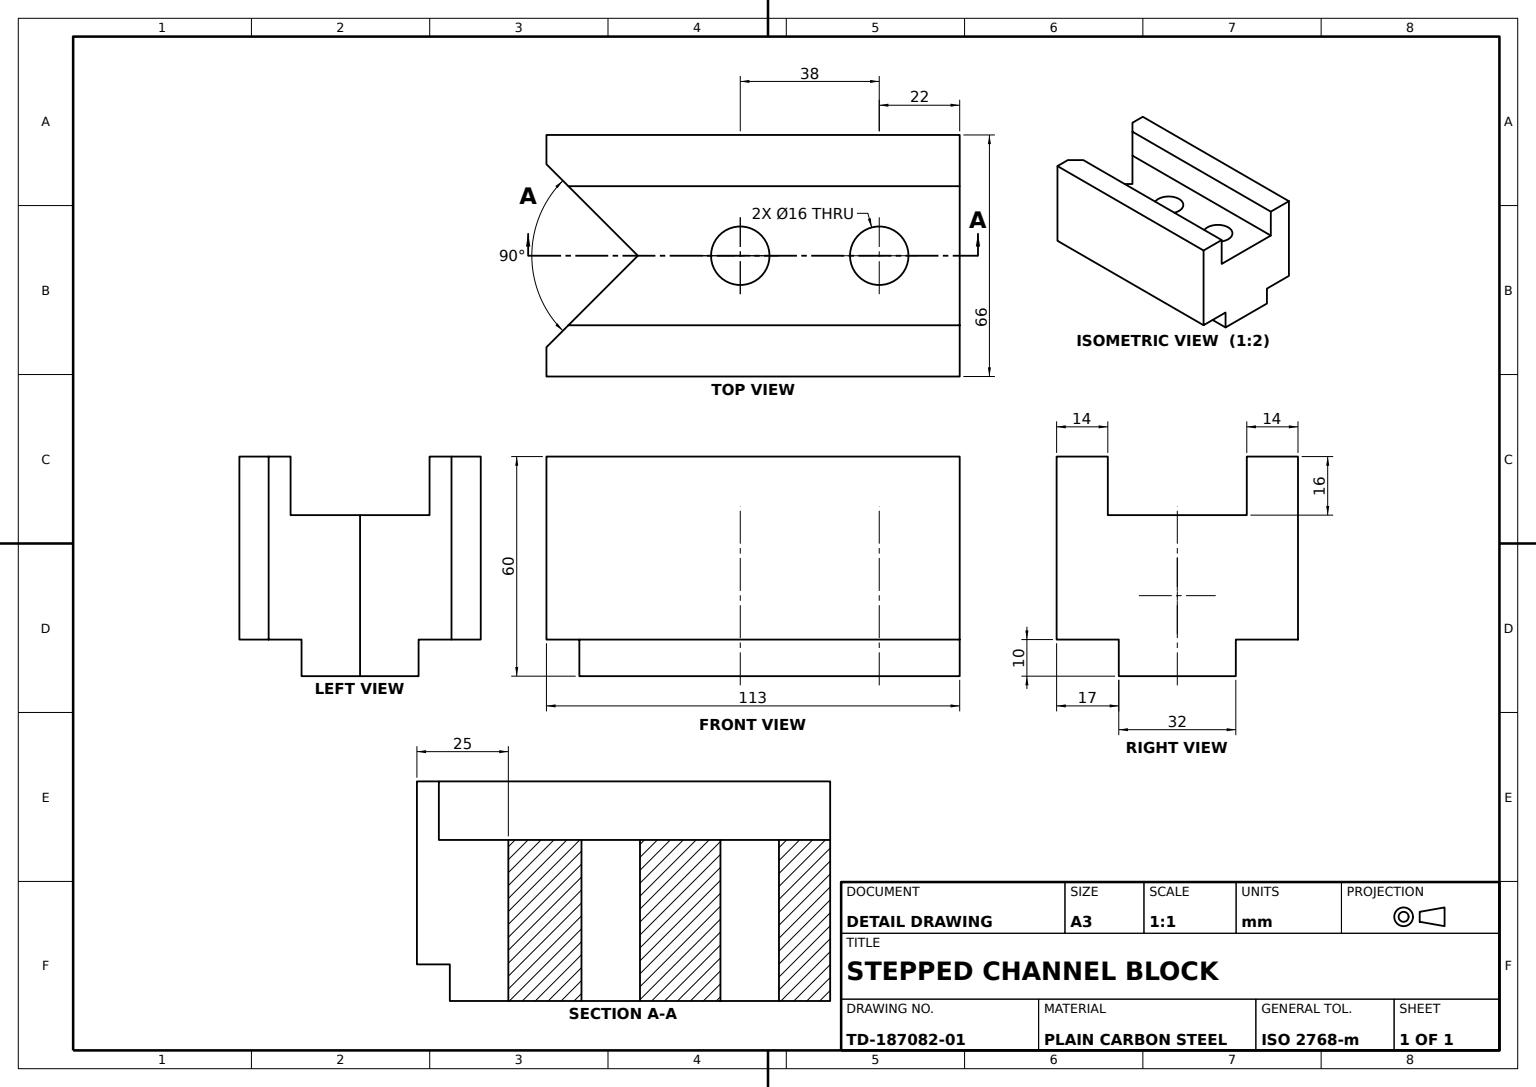
from build123d import *

# Parameters (mm, degrees)
CHANNEL_BLOCK_DEPTH       = 56.5
THROUGH_HOLES_SKETCH_R    = 8
THROUGH_HOLES_2X_16_DEPTH = 98.387114137
SIDE_CUT_DEPTH            = 101.240959692
SIDE_CUT_DEPTH_BACK       = 101.240959692


with BuildPart() as part:
    # Channel Profile Sketch → Channel Block (new, symmetric)
    with BuildSketch(Plane.XY):
        Polygon((0, 0), (0, 50), (14, 50), (14, 34), (52, 34), (52, 50), (66, 50), (66, 0), (49, 0), (49, -10), (17, -10), (17, 0), align=None)
    extrude(amount=CHANNEL_BLOCK_DEPTH, both=True)

    # Through Holes Sketch → Through Holes 2xØ16 (cut, through all)
    with BuildSketch(Plane(origin=(0, 34, 0), x_dir=(1, 0, 0), z_dir=(0, 1, 0))):
        with Locations(Location((33, 34.5, 0), (0, 0, 270))):
            Circle(THROUGH_HOLES_SKETCH_R)
        with Locations(Location((33, -3.5, 0), (0, 0, 270))):
            Circle(THROUGH_HOLES_SKETCH_R)
    extrude(amount=-THROUGH_HOLES_2X_16_DEPTH, mode=Mode.SUBTRACT)

    # Side Cut Sketch → Side Cut (cut, two sides: drawn at the far end of the back side and taken through both)
    with BuildSketch(Plane(origin=(0, 0, 0), x_dir=(1, 0, 0), z_dir=(0, 1, 0)).offset(-SIDE_CUT_DEPTH_BACK)):
        Polygon((-178.698459932, -243.198459932), (8, -56.5), (33, -31.5), (58, -56.5), (244.698459932, -243.198459932), (244.698459932, -771.261448153), (-178.698459932, -771.261448153), align=None)
    extrude(amount=SIDE_CUT_DEPTH + SIDE_CUT_DEPTH_BACK, mode=Mode.SUBTRACT)


solid = part.part
